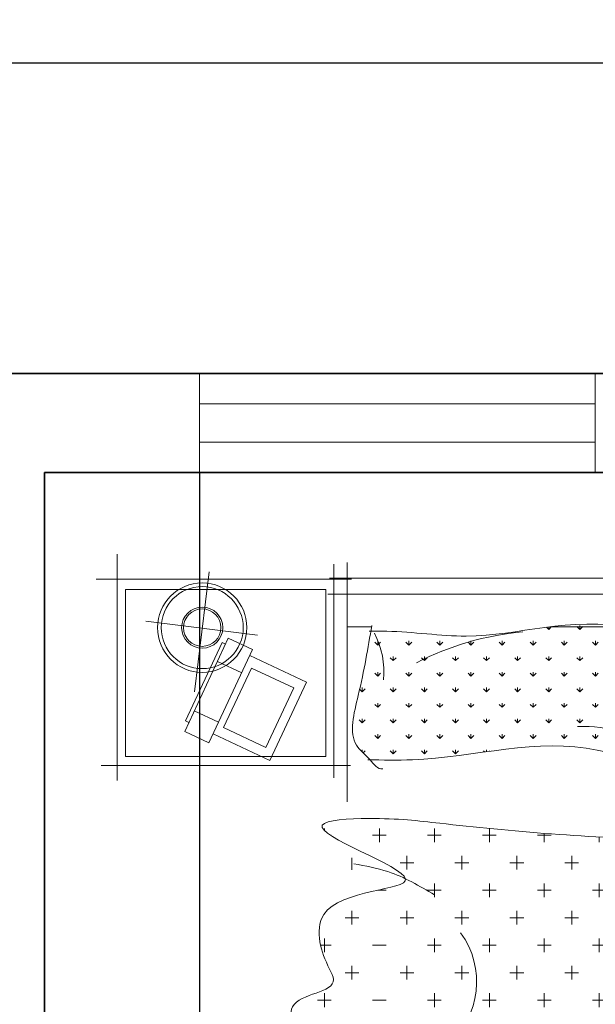
# Model space of a CAD drawing. Units: inches. Extents: x -26 to 575, y -18 to 513.
# Tile 13 of 28: x 136 to 189, y 418 to 508. Entities that reach past the tile are written whole.
import ezdxf

# ---------------------------------------------------------------- set-up
doc = ezdxf.new("R2010")
doc.units = ezdxf.units.IN
doc.header["$MEASUREMENT"] = 0
for name, color, linetype, lineweight in [('A-ANNO-DIMS', 2, 'Continuous', 18), ('A-GLAZ', 4, 'Continuous', 18), ('A-WALL', 7, 'Continuous', 35), ('Furniture', 8, 'Continuous', 15)]:
    doc.layers.add(name, color=color, linetype=linetype, lineweight=lineweight)
doc.styles.get("Standard").update_dxf_attribs({"font": 'arial.ttf', "height": 6})
doc.dimstyles.get("Standard").update_dxf_attribs({"dimtxt": 6, "dimasz": 0.18, "dimexe": 0.18, "dimexo": 0.0625, "dimgap": 0.09, "dimtad": 0, "dimtih": 1, "dimtoh": 1, "dimzin": 0, "dimdsep": 46, "dimlunit": 3, "dimtxsty": 'Standard', "dimcen": 0.09, "dimadec": 0, "dimazin": 0, "dimtfac": 1, "dimtofl": 0, "dimtmove": 0, "dimatfit": 3, "dimfxl": 1, "dimtolj": 1, "dimtzin": 0, "dimarcsym": 0})

# ---------------------------------------------------------------- blocks, each defined once
blk = doc.blocks.new('*D1')
at = {"layer": 'A-ANNO-DIMS', "color": 0, "lineweight": -2, "transparency": 16777216}
for p, q in [((18.177, 475.57), (18.177, 503.937)), ((18.357, 503.757), (264.875, 503.757)), ((521.997, 503.757), (275.479, 503.757)), ((522.177, 475.57), (522.177, 503.937))]:
    blk.add_line(p, q, dxfattribs=at)
at = {"layer": 'A-ANNO-DIMS', "color": 0, "transparency": 16777216}
for points in [[(18.357, 503.787), (18.357, 503.727), (18.177, 503.757)], [(521.997, 503.787), (521.997, 503.727), (522.177, 503.757)]]:
    blk.add_solid(points, dxfattribs=at)
at = {"layer": 'Defpoints', "color": 0, "transparency": 16777216}
for p in [(522.177, 503.757), (18.177, 475.508), (522.177, 475.508)]:
    blk.add_point(p, dxfattribs=at)
at = {"layer": 'A-ANNO-DIMS', "color": 0, "transparency": 16777216, "insert": (270.177, 503.757), "char_height": 6, "attachment_point": 5}
blk.add_mtext("\\A1;42'", dxfattribs=at)
blk = doc.blocks.new('BED-DOUBLE-WITH-NIGHTSTANDS')
for p, q in [((1.925, 83.361), (1.925, 62.761)), ((82.669, 83.361), (82.669, 62.761)), ((21.61, 63.031), (21.61, 82.461)), ((22.828, 60.828), (22.828, 82.615)), ((102.354, 63.031), (102.354, 82.461)), ((10.269, 81.761), (8.938, 70.826)), ((81.883, 82.344), (81.883, 56.232)), ((23.226, 81.078), (0, 81.078)), ((21.24, 81.17), (81.883, 81.17)), ((103.97, 81.078), (80.744, 81.078)), ((20.889, 80.153), (2.667, 80.153)), ((2.667, 80.153), (2.667, 64.968)), ((20.889, 64.968), (20.889, 80.153)), ((82.669, 79.717), (21.062, 79.717)), ((101.633, 80.153), (83.411, 80.153)), ((83.411, 80.153), (83.411, 64.968)), ((101.633, 64.968), (101.633, 80.153)), ((92.567, 79.403), (92.567, 67.508)), ((14.667, 76.005), (4.51, 77.257)), ((25.057, 76.764), (22.828, 76.764)), ((41.168, 76.507), (40.96, 76.715)), ((41.168, 76.507), (41.434, 76.772)), ((41.169, 76.507), (41.169, 76.741)), ((56.226, 76.764), (41.357, 76.764)), ((43.997, 76.507), (43.732, 76.772)), ((43.997, 76.507), (43.997, 76.882)), ((43.997, 76.507), (44.262, 76.772)), ((46.825, 76.507), (46.56, 76.772)), ((46.825, 76.507), (47.09, 76.772)), ((46.826, 76.507), (46.826, 76.882)), ((57.003, 76.507), (56.737, 76.772)), ((57.003, 76.507), (57.003, 76.828)), ((57.003, 76.507), (57.268, 76.772)), ((81.883, 76.764), (59.394, 76.764)), ((59.831, 76.507), (59.594, 76.744)), ((59.831, 76.507), (59.831, 76.717)), ((59.831, 76.507), (60.018, 76.694)), ((8.056, 67.244), (12.026, 75.725)), ((11.458, 75.323), (8.122, 68.196)), ((11.769, 75.177), (11.458, 75.323)), ((12.026, 75.725), (14.235, 74.691)), ((25.612, 75.093), (25.347, 75.358)), ((25.612, 75.093), (25.612, 75.468)), ((25.612, 75.093), (25.877, 75.358)), ((28.44, 75.093), (28.175, 75.358)), ((28.44, 75.093), (28.706, 75.358)), ((28.441, 75.093), (28.441, 75.468)), ((31.269, 75.093), (31.004, 75.358)), ((31.269, 75.093), (31.269, 75.468)), ((31.269, 75.093), (31.534, 75.358)), ((34.097, 75.093), (33.832, 75.358)), ((34.097, 75.093), (34.362, 75.358)), ((34.098, 75.093), (34.098, 75.468)), ((36.926, 75.093), (36.661, 75.358)), ((36.926, 75.093), (36.926, 75.468)), ((36.926, 75.093), (37.191, 75.358)), ((39.754, 75.093), (39.489, 75.358)), ((39.754, 75.093), (40.019, 75.358)), ((39.755, 75.093), (39.755, 75.468)), ((42.583, 75.093), (42.317, 75.358)), ((42.583, 75.093), (42.583, 75.468)), ((42.583, 75.093), (42.848, 75.358)), ((45.411, 75.093), (45.146, 75.358)), ((45.411, 75.093), (45.411, 75.468)), ((45.411, 75.093), (45.676, 75.358)), ((48.239, 75.093), (47.974, 75.358)), ((48.239, 75.093), (48.505, 75.358)), ((48.24, 75.093), (48.24, 75.468)), ((51.068, 75.093), (50.803, 75.358)), ((53.004, 75.337), (53.025, 75.358)), ((55.588, 75.093), (55.323, 75.358)), ((55.588, 75.093), (55.854, 75.358)), ((55.589, 75.093), (55.589, 75.468)), ((58.417, 75.093), (58.152, 75.358)), ((58.417, 75.093), (58.417, 75.468)), ((58.417, 75.093), (58.682, 75.358)), ((61.245, 75.093), (60.98, 75.358)), ((61.245, 75.093), (61.51, 75.358)), ((61.246, 75.093), (61.246, 75.468)), ((64.074, 75.093), (63.809, 75.358)), ((64.074, 75.093), (64.074, 75.468)), ((64.074, 75.093), (64.339, 75.358)), ((66.902, 75.093), (66.637, 75.358)), ((66.902, 75.093), (67.167, 75.358)), ((66.903, 75.093), (66.903, 75.468)), ((69.731, 75.093), (69.465, 75.358)), ((69.731, 75.093), (69.731, 75.468)), ((69.731, 75.093), (69.996, 75.358)), ((72.559, 75.093), (72.294, 75.358)), ((72.559, 75.093), (72.559, 75.468)), ((72.559, 75.093), (72.824, 75.358)), ((75.387, 75.093), (75.122, 75.358)), ((75.387, 75.093), (75.653, 75.358)), ((75.388, 75.093), (75.388, 75.468)), ((78.216, 75.093), (77.951, 75.358)), ((78.216, 75.093), (78.216, 75.468)), ((78.216, 75.093), (78.481, 75.358)), ((14.235, 74.691), (10.265, 66.21)), ((51.068, 75.093), (51.068, 75.099)), ((51.068, 75.093), (51.07, 75.095)), ((13.242, 72.571), (11.033, 73.605)), ((19.14, 71.727), (13.978, 74.143)), ((27.026, 73.679), (26.761, 73.944)), ((27.026, 73.679), (27.291, 73.944)), ((27.027, 73.678), (27.027, 74.053)), ((29.855, 73.679), (29.589, 73.944)), ((29.855, 73.678), (29.855, 74.053)), ((29.855, 73.679), (30.12, 73.944)), ((32.683, 73.679), (32.418, 73.944)), ((32.683, 73.678), (32.683, 74.053)), ((32.683, 73.679), (32.948, 73.944)), ((35.512, 73.679), (35.246, 73.944)), ((35.512, 73.678), (35.512, 74.053)), ((35.512, 73.679), (35.777, 73.944)), ((38.34, 73.679), (38.075, 73.944)), ((38.34, 73.678), (38.34, 74.053)), ((38.34, 73.679), (38.605, 73.944)), ((41.168, 73.679), (40.903, 73.944)), ((41.168, 73.679), (41.434, 73.944)), ((41.169, 73.678), (41.169, 74.053)), ((43.997, 73.679), (43.732, 73.944)), ((43.997, 73.678), (43.997, 74.053)), ((43.997, 73.679), (44.262, 73.944)), ((46.825, 73.679), (46.56, 73.944)), ((46.825, 73.679), (47.09, 73.944)), ((46.826, 73.678), (46.826, 74.053)), ((49.654, 73.679), (49.388, 73.944)), ((49.654, 73.678), (49.654, 74.053)), ((49.654, 73.679), (49.919, 73.944)), ((54.174, 73.679), (53.909, 73.944)), ((54.174, 73.679), (54.439, 73.944)), ((54.175, 73.678), (54.175, 74.053)), ((57.003, 73.679), (56.737, 73.944)), ((57.003, 73.678), (57.003, 74.053)), ((57.003, 73.679), (57.268, 73.944)), ((59.831, 73.679), (59.566, 73.944)), ((59.831, 73.678), (59.831, 74.053)), ((59.831, 73.679), (60.096, 73.944)), ((62.66, 73.679), (62.394, 73.944)), ((62.66, 73.678), (62.66, 74.053)), ((62.66, 73.679), (62.925, 73.944)), ((65.488, 73.679), (65.223, 73.944)), ((65.488, 73.678), (65.488, 74.053)), ((65.488, 73.679), (65.753, 73.944)), ((68.316, 73.679), (68.051, 73.944)), ((68.316, 73.679), (68.582, 73.944)), ((68.317, 73.678), (68.317, 74.053)), ((71.145, 73.679), (70.88, 73.944)), ((71.145, 73.678), (71.145, 74.053)), ((71.145, 73.679), (71.41, 73.944)), ((73.973, 73.679), (73.708, 73.944)), ((73.973, 73.679), (74.238, 73.944)), ((73.974, 73.678), (73.974, 74.053)), ((76.802, 73.679), (76.536, 73.944)), ((76.802, 73.678), (76.802, 74.053)), ((76.802, 73.679), (77.067, 73.944)), ((79.63, 73.679), (79.365, 73.944)), ((79.63, 73.678), (79.63, 74.053)), ((79.63, 73.679), (79.895, 73.944)), ((14.129, 73), (11.598, 67.591)), ((17.984, 71.195), (14.129, 73)), ((25.612, 72.264), (25.612, 72.639)), ((28.441, 72.264), (28.441, 72.639)), ((31.269, 72.264), (31.269, 72.639)), ((34.098, 72.264), (34.098, 72.639)), ((36.926, 72.264), (36.926, 72.639)), ((39.755, 72.264), (39.755, 72.639)), ((42.583, 72.264), (42.583, 72.639)), ((45.411, 72.264), (45.411, 72.639)), ((48.24, 72.264), (48.24, 72.639)), ((55.589, 72.264), (55.589, 72.639)), ((58.417, 72.264), (58.417, 72.639)), ((61.246, 72.264), (61.246, 72.639)), ((64.074, 72.264), (64.074, 72.639)), ((66.903, 72.264), (66.903, 72.639)), ((69.731, 72.264), (69.731, 72.639)), ((72.559, 72.264), (72.559, 72.639)), ((75.388, 72.264), (75.388, 72.639)), ((78.216, 72.264), (78.216, 72.639)), ((98.466, 73.144), (86.668, 73.144)), ((15.804, 64.601), (19.14, 71.727)), ((25.612, 72.265), (25.347, 72.53)), ((25.612, 72.265), (25.877, 72.53)), ((28.44, 72.265), (28.175, 72.53)), ((28.44, 72.265), (28.706, 72.53)), ((31.269, 72.265), (31.004, 72.53)), ((31.269, 72.265), (31.534, 72.53)), ((34.097, 72.265), (33.832, 72.53)), ((34.097, 72.265), (34.362, 72.53)), ((36.926, 72.265), (36.661, 72.53)), ((36.926, 72.265), (37.191, 72.53)), ((39.754, 72.265), (39.489, 72.53)), ((39.754, 72.265), (40.019, 72.53)), ((42.583, 72.265), (42.317, 72.53)), ((42.583, 72.265), (42.848, 72.53)), ((45.411, 72.265), (45.146, 72.53)), ((45.411, 72.265), (45.676, 72.53)), ((48.239, 72.265), (47.974, 72.53)), ((48.239, 72.265), (48.505, 72.53)), ((55.588, 72.265), (55.323, 72.53)), ((55.588, 72.265), (55.854, 72.53)), ((58.417, 72.265), (58.152, 72.53)), ((58.417, 72.265), (58.682, 72.53)), ((61.245, 72.265), (60.98, 72.53)), ((61.245, 72.265), (61.51, 72.53)), ((64.074, 72.265), (63.809, 72.53)), ((64.074, 72.265), (64.339, 72.53)), ((66.902, 72.265), (66.637, 72.53)), ((66.902, 72.265), (67.167, 72.53)), ((69.731, 72.265), (69.465, 72.53)), ((69.731, 72.265), (69.996, 72.53)), ((72.559, 72.265), (72.294, 72.53)), ((72.559, 72.265), (72.824, 72.53)), ((75.387, 72.265), (75.122, 72.53)), ((75.387, 72.265), (75.653, 72.53)), ((78.216, 72.265), (77.951, 72.53)), ((78.216, 72.265), (78.481, 72.53)), ((15.452, 65.787), (17.984, 71.195)), ((24.198, 70.85), (23.972, 71.076)), ((24.198, 70.85), (24.198, 71.225)), ((24.198, 70.85), (24.463, 71.116)), ((27.026, 70.85), (26.761, 71.116)), ((27.026, 70.85), (27.291, 71.116)), ((27.027, 70.85), (27.027, 71.225)), ((29.855, 70.85), (29.589, 71.116)), ((29.855, 70.85), (29.855, 71.225)), ((29.855, 70.85), (30.12, 71.116)), ((32.683, 70.85), (32.418, 71.116)), ((32.683, 70.85), (32.683, 71.225)), ((32.683, 70.85), (32.948, 71.116)), ((35.512, 70.85), (35.246, 71.116)), ((35.512, 70.85), (35.512, 71.225)), ((35.512, 70.85), (35.777, 71.116)), ((38.34, 70.85), (38.075, 71.116)), ((38.34, 70.85), (38.34, 71.225)), ((38.34, 70.85), (38.605, 71.116)), ((41.168, 70.85), (40.903, 71.116)), ((41.168, 70.85), (41.434, 71.116)), ((41.169, 70.85), (41.169, 71.225)), ((43.997, 70.85), (43.732, 71.116)), ((43.997, 70.85), (43.997, 71.225)), ((43.997, 70.85), (44.262, 71.116)), ((46.825, 70.85), (46.56, 71.116)), ((46.825, 70.85), (47.09, 71.116)), ((46.826, 70.85), (46.826, 71.225)), ((49.654, 70.85), (49.388, 71.116)), ((49.654, 70.85), (49.654, 71.225)), ((49.654, 70.85), (49.919, 71.116)), ((54.174, 70.85), (53.909, 71.116)), ((54.174, 70.85), (54.439, 71.116)), ((54.175, 70.85), (54.175, 71.225)), ((57.003, 70.85), (56.737, 71.116)), ((57.003, 70.85), (57.003, 71.225)), ((57.003, 70.85), (57.268, 71.116)), ((59.831, 70.85), (59.566, 71.116)), ((59.831, 70.85), (59.831, 71.225)), ((59.831, 70.85), (60.096, 71.116)), ((62.66, 70.85), (62.394, 71.116)), ((62.66, 70.85), (62.66, 71.225)), ((62.66, 70.85), (62.925, 71.116)), ((65.488, 70.85), (65.223, 71.116)), ((65.488, 70.85), (65.488, 71.225)), ((65.488, 70.85), (65.753, 71.116)), ((68.316, 70.85), (68.051, 71.116)), ((68.316, 70.85), (68.582, 71.116)), ((68.317, 70.85), (68.317, 71.225)), ((71.145, 70.85), (70.88, 71.116)), ((71.145, 70.85), (71.145, 71.225)), ((71.145, 70.85), (71.41, 71.116)), ((73.973, 70.85), (73.708, 71.116)), ((73.973, 70.85), (74.238, 71.116)), ((73.974, 70.85), (73.974, 71.225)), ((76.802, 70.85), (76.536, 71.116)), ((76.802, 70.85), (76.802, 71.225)), ((76.802, 70.85), (77.067, 71.116)), ((79.63, 70.85), (79.365, 71.116)), ((79.63, 70.85), (79.63, 71.225)), ((79.63, 70.85), (79.895, 71.116)), ((11.136, 68.071), (8.927, 69.105)), ((25.612, 69.436), (25.347, 69.701)), ((25.612, 69.436), (25.612, 69.811)), ((25.612, 69.436), (25.877, 69.701)), ((28.44, 69.436), (28.175, 69.701)), ((28.44, 69.436), (28.706, 69.701)), ((28.441, 69.436), (28.441, 69.811)), ((31.269, 69.436), (31.004, 69.701)), ((31.269, 69.436), (31.269, 69.811)), ((31.269, 69.436), (31.534, 69.701)), ((34.097, 69.436), (33.832, 69.701)), ((34.097, 69.436), (34.362, 69.701)), ((34.098, 69.436), (34.098, 69.811)), ((36.926, 69.436), (36.661, 69.701)), ((36.926, 69.436), (36.926, 69.811)), ((36.926, 69.436), (37.191, 69.701)), ((39.754, 69.436), (39.489, 69.701)), ((39.754, 69.436), (40.019, 69.701)), ((39.755, 69.436), (39.755, 69.811)), ((42.583, 69.436), (42.317, 69.701)), ((42.583, 69.436), (42.583, 69.811)), ((42.583, 69.436), (42.848, 69.701)), ((45.411, 69.436), (45.146, 69.701)), ((45.411, 69.436), (45.411, 69.811)), ((45.411, 69.436), (45.676, 69.701)), ((48.239, 69.436), (47.974, 69.701)), ((48.239, 69.436), (48.505, 69.701)), ((48.24, 69.436), (48.24, 69.811)), ((51.052, 69.452), (50.803, 69.701)), ((53.007, 69.683), (53.025, 69.701)), ((55.588, 69.436), (55.323, 69.701)), ((55.588, 69.436), (55.854, 69.701)), ((55.589, 69.436), (55.589, 69.811)), ((58.417, 69.436), (58.152, 69.701)), ((58.417, 69.436), (58.417, 69.811)), ((58.417, 69.436), (58.682, 69.701)), ((61.245, 69.436), (60.98, 69.701)), ((61.245, 69.436), (61.51, 69.701)), ((61.246, 69.436), (61.246, 69.811)), ((64.074, 69.436), (63.809, 69.701)), ((64.074, 69.436), (64.074, 69.811)), ((64.074, 69.436), (64.339, 69.701)), ((66.902, 69.436), (66.637, 69.701)), ((66.902, 69.436), (67.167, 69.701)), ((66.903, 69.436), (66.903, 69.811)), ((69.731, 69.436), (69.465, 69.701)), ((69.731, 69.436), (69.731, 69.811)), ((69.731, 69.436), (69.996, 69.701)), ((72.559, 69.436), (72.294, 69.701)), ((72.559, 69.436), (72.559, 69.811)), ((72.559, 69.436), (72.824, 69.701)), ((75.387, 69.436), (75.122, 69.701)), ((75.387, 69.436), (75.653, 69.701)), ((75.388, 69.436), (75.388, 69.811)), ((78.216, 69.436), (77.951, 69.701)), ((78.216, 69.436), (78.216, 69.811)), ((78.216, 69.436), (78.481, 69.701)), ((8.122, 68.196), (8.434, 68.05)), ((24.198, 68.022), (23.933, 68.287)), ((24.198, 68.022), (24.198, 68.397)), ((24.198, 68.022), (24.463, 68.287)), ((27.026, 68.022), (26.761, 68.287)), ((27.026, 68.022), (27.291, 68.287)), ((27.027, 68.022), (27.027, 68.397)), ((29.855, 68.022), (29.589, 68.287)), ((29.855, 68.022), (29.855, 68.397)), ((29.855, 68.022), (30.12, 68.287)), ((32.683, 68.022), (32.418, 68.287)), ((32.683, 68.022), (32.683, 68.397)), ((32.683, 68.022), (32.948, 68.287)), ((35.512, 68.022), (35.246, 68.287)), ((35.512, 68.022), (35.512, 68.397)), ((35.512, 68.022), (35.777, 68.287)), ((38.34, 68.022), (38.075, 68.287)), ((38.34, 68.022), (38.34, 68.397)), ((38.34, 68.022), (38.605, 68.287)), ((41.168, 68.022), (40.903, 68.287)), ((41.168, 68.022), (41.434, 68.287)), ((41.169, 68.022), (41.169, 68.397)), ((43.997, 68.022), (43.732, 68.287)), ((43.997, 68.022), (43.997, 68.397)), ((43.997, 68.022), (44.262, 68.287)), ((46.825, 68.022), (46.56, 68.287)), ((46.825, 68.022), (47.09, 68.287)), ((46.826, 68.022), (46.826, 68.397)), ((49.654, 68.022), (49.388, 68.287)), ((49.654, 68.022), (49.654, 68.397)), ((49.654, 68.022), (49.919, 68.287)), ((54.174, 68.022), (53.909, 68.287)), ((54.174, 68.022), (54.439, 68.287)), ((54.175, 68.022), (54.175, 68.397)), ((57.003, 68.022), (56.737, 68.287)), ((57.003, 68.022), (57.003, 68.397)), ((57.003, 68.022), (57.268, 68.287)), ((59.831, 68.022), (59.566, 68.287)), ((59.831, 68.022), (59.831, 68.397)), ((59.831, 68.022), (60.096, 68.287)), ((62.66, 68.022), (62.394, 68.287)), ((62.66, 68.022), (62.66, 68.397)), ((62.66, 68.022), (62.925, 68.287)), ((65.488, 68.022), (65.223, 68.287)), ((65.488, 68.022), (65.488, 68.397)), ((65.488, 68.022), (65.753, 68.287)), ((68.316, 68.022), (68.051, 68.287)), ((68.316, 68.022), (68.582, 68.287)), ((68.317, 68.022), (68.317, 68.397)), ((71.145, 68.022), (70.88, 68.287)), ((71.145, 68.022), (71.145, 68.397)), ((71.145, 68.022), (71.41, 68.287)), ((73.973, 68.022), (73.708, 68.287)), ((73.973, 68.022), (74.238, 68.287)), ((73.974, 68.022), (73.974, 68.397)), ((76.802, 68.022), (76.536, 68.287)), ((76.802, 68.022), (76.802, 68.397)), ((76.802, 68.022), (77.067, 68.287)), ((79.63, 68.022), (79.365, 68.287)), ((79.63, 68.022), (79.63, 68.397)), ((79.63, 68.022), (79.895, 68.287)), ((10.265, 66.21), (8.056, 67.244)), ((11.598, 67.591), (15.452, 65.787)), ((10.642, 67.017), (15.804, 64.601)), ((25.612, 66.608), (25.347, 66.873)), ((25.612, 66.607), (25.612, 66.982)), ((25.612, 66.608), (25.877, 66.873)), ((28.44, 66.608), (28.175, 66.873)), ((28.44, 66.608), (28.706, 66.873)), ((28.441, 66.607), (28.441, 66.982)), ((31.269, 66.608), (31.004, 66.873)), ((31.269, 66.607), (31.269, 66.982)), ((31.269, 66.608), (31.534, 66.873)), ((34.097, 66.608), (33.832, 66.873)), ((34.097, 66.608), (34.362, 66.873)), ((34.098, 66.607), (34.098, 66.982)), ((36.926, 66.608), (36.661, 66.873)), ((36.926, 66.607), (36.926, 66.982)), ((36.926, 66.608), (37.191, 66.873)), ((39.754, 66.608), (39.489, 66.873)), ((39.754, 66.608), (40.019, 66.873)), ((39.755, 66.607), (39.755, 66.982)), ((42.583, 66.608), (42.317, 66.873)), ((42.583, 66.607), (42.583, 66.982)), ((42.583, 66.608), (42.848, 66.873)), ((45.411, 66.608), (45.146, 66.873)), ((45.411, 66.607), (45.411, 66.982)), ((45.411, 66.608), (45.676, 66.873)), ((48.239, 66.608), (47.974, 66.873)), ((48.239, 66.608), (48.505, 66.873)), ((48.24, 66.607), (48.24, 66.982)), ((51.068, 66.608), (50.803, 66.873)), ((51.068, 66.607), (51.068, 66.982)), ((51.068, 66.608), (51.333, 66.873)), ((52.76, 66.608), (52.495, 66.873)), ((52.76, 66.607), (52.76, 66.982)), ((52.76, 66.608), (53.025, 66.873)), ((55.588, 66.608), (55.323, 66.873)), ((55.588, 66.608), (55.854, 66.873)), ((55.589, 66.607), (55.589, 66.982)), ((58.417, 66.608), (58.152, 66.873)), ((58.417, 66.607), (58.417, 66.982)), ((58.417, 66.608), (58.682, 66.873)), ((61.245, 66.608), (60.98, 66.873)), ((61.245, 66.608), (61.51, 66.873)), ((61.246, 66.607), (61.246, 66.982)), ((64.074, 66.608), (63.809, 66.873)), ((64.074, 66.607), (64.074, 66.982)), ((64.074, 66.608), (64.339, 66.873)), ((66.902, 66.608), (66.637, 66.873)), ((66.902, 66.608), (67.167, 66.873)), ((66.903, 66.607), (66.903, 66.982)), ((69.731, 66.608), (69.465, 66.873)), ((69.731, 66.607), (69.731, 66.982)), ((69.731, 66.608), (69.996, 66.873)), ((72.559, 66.608), (72.294, 66.873)), ((72.559, 66.607), (72.559, 66.982)), ((72.559, 66.608), (72.824, 66.873)), ((75.387, 66.608), (75.122, 66.873)), ((75.387, 66.608), (75.653, 66.873)), ((75.388, 66.607), (75.388, 66.982)), ((78.216, 66.608), (77.951, 66.873)), ((78.216, 66.607), (78.216, 66.982)), ((78.216, 66.608), (78.481, 66.873)), ((81.044, 66.608), (80.779, 66.873)), ((81.044, 66.608), (81.253, 66.817)), ((81.045, 66.607), (81.045, 66.982)), ((24.198, 65.385), (24.198, 65.568)), ((24.295, 65.291), (24.463, 65.459)), ((27.026, 65.194), (26.761, 65.459)), ((27.026, 65.194), (27.291, 65.459)), ((27.027, 65.193), (27.027, 65.568)), ((29.855, 65.194), (29.589, 65.459)), ((29.855, 65.193), (29.855, 65.568)), ((29.855, 65.194), (30.12, 65.459)), ((32.683, 65.194), (32.418, 65.459)), ((32.683, 65.193), (32.683, 65.568)), ((32.683, 65.194), (32.948, 65.459)), ((35.335, 65.37), (35.246, 65.459)), ((35.512, 65.394), (35.512, 65.568)), ((35.743, 65.425), (35.777, 65.459)), ((46.774, 65.245), (46.56, 65.459)), ((46.826, 65.232), (46.826, 65.568)), ((46.856, 65.224), (47.09, 65.459)), ((49.654, 65.194), (49.388, 65.459)), ((49.654, 65.193), (49.654, 65.568)), ((49.654, 65.194), (49.919, 65.459)), ((54.174, 65.194), (53.909, 65.459)), ((54.174, 65.194), (54.439, 65.459)), ((54.175, 65.193), (54.175, 65.568)), ((57.003, 65.194), (56.737, 65.459)), ((57.003, 65.193), (57.003, 65.568)), ((57.003, 65.194), (57.268, 65.459)), ((59.831, 65.194), (59.566, 65.459)), ((59.831, 65.193), (59.831, 65.568)), ((59.831, 65.194), (60.096, 65.459)), ((62.66, 65.525), (62.66, 65.568)), ((65.488, 65.481), (65.488, 65.568)), ((65.74, 65.446), (65.753, 65.459)), ((68.316, 65.194), (68.051, 65.459)), ((68.316, 65.194), (68.582, 65.459)), ((68.317, 65.193), (68.317, 65.568)), ((71.145, 65.194), (70.88, 65.459)), ((71.145, 65.193), (71.145, 65.568)), ((71.145, 65.194), (71.41, 65.459)), ((73.973, 65.194), (73.708, 65.459)), ((73.973, 65.194), (74.238, 65.459)), ((73.974, 65.193), (73.974, 65.568)), ((76.802, 65.194), (76.536, 65.459)), ((76.802, 65.193), (76.802, 65.568)), ((76.802, 65.194), (77.067, 65.459)), ((79.63, 65.194), (79.365, 65.459)), ((79.63, 65.193), (79.63, 65.568)), ((79.63, 65.194), (79.895, 65.459)), ((82.154, 61.735), (82.154, 65.422)), ((2.667, 64.968), (20.889, 64.968)), ((83.411, 64.968), (101.633, 64.968)), ((0.451, 64.149), (23.136, 64.149)), ((55.589, 64.121), (55.589, 64.154)), ((81.194, 64.149), (103.88, 64.149)), ((78.267, 59.667), (78.267, 60.149)), ((20.767, 58.212), (20.767, 58.417)), ((25.767, 57.167), (25.767, 58.417)), ((30.767, 57.167), (30.767, 58.417)), ((35.767, 57.167), (35.767, 58.407)), ((70.767, 57.167), (70.767, 58.417)), ((75.767, 57.167), (75.767, 58.417)), ((80.767, 57.167), (80.767, 58.417)), ((21.392, 57.792), (21.312, 57.792)), ((26.392, 57.792), (25.142, 57.792)), ((31.392, 57.792), (30.142, 57.792)), ((36.392, 57.792), (35.142, 57.792)), ((41.392, 57.792), (40.142, 57.792)), ((40.767, 57.167), (40.767, 57.965)), ((45.767, 57.167), (45.767, 57.639)), ((50.767, 57.167), (50.767, 57.462)), ((55.767, 57.167), (55.767, 57.483)), ((60.767, 57.167), (60.767, 57.735)), ((66.392, 57.792), (65.142, 57.792)), ((65.767, 57.167), (65.767, 58.213)), ((71.392, 57.792), (70.142, 57.792)), ((76.392, 57.792), (75.142, 57.792)), ((81.392, 57.792), (80.142, 57.792)), ((23.273, 54.636), (23.273, 55.755)), ((28.267, 54.667), (28.267, 55.917)), ((33.267, 54.667), (33.267, 55.917)), ((38.267, 54.667), (38.267, 55.917)), ((43.267, 54.667), (43.267, 55.917)), ((48.267, 54.667), (48.267, 55.917)), ((53.267, 54.667), (53.267, 55.917)), ((58.267, 54.667), (58.267, 55.917)), ((63.267, 54.667), (63.267, 55.917)), ((68.267, 54.667), (68.267, 55.917)), ((73.267, 54.667), (73.267, 55.917)), ((78.267, 54.667), (78.267, 55.917)), ((83.267, 54.667), (83.267, 55.917)), ((28.892, 55.292), (27.642, 55.292)), ((33.892, 55.292), (32.642, 55.292)), ((38.892, 55.292), (37.642, 55.292)), ((43.892, 55.292), (42.642, 55.292)), ((48.892, 55.292), (47.642, 55.292)), ((53.892, 55.292), (52.642, 55.292)), ((58.892, 55.292), (57.642, 55.292)), ((63.892, 55.292), (62.642, 55.292)), ((68.892, 55.292), (67.642, 55.292)), ((73.892, 55.292), (72.642, 55.292)), ((78.892, 55.292), (77.642, 55.292)), ((83.892, 55.292), (82.642, 55.292)), ((30.767, 52.167), (30.767, 53.417)), ((35.767, 52.167), (35.767, 53.417)), ((40.767, 52.167), (40.767, 53.417)), ((45.767, 52.167), (45.767, 53.417)), ((50.767, 52.167), (50.767, 53.417)), ((55.767, 52.167), (55.767, 53.417)), ((60.767, 52.167), (60.767, 53.417)), ((65.767, 52.167), (65.767, 53.417)), ((70.767, 52.167), (70.767, 53.417)), ((75.767, 52.167), (75.767, 53.417)), ((80.767, 52.167), (80.767, 53.417)), ((26.392, 52.792), (25.619, 52.792)), ((31.392, 52.792), (30.142, 52.792)), ((36.392, 52.792), (35.142, 52.792)), ((41.392, 52.792), (40.142, 52.792)), ((46.392, 52.792), (45.142, 52.792)), ((51.392, 52.792), (50.142, 52.792)), ((56.392, 52.792), (55.142, 52.792)), ((61.392, 52.792), (60.142, 52.792)), ((66.392, 52.792), (65.142, 52.792)), ((71.392, 52.792), (70.142, 52.792)), ((76.392, 52.792), (75.142, 52.792)), ((81.392, 52.792), (80.142, 52.792)), ((23.892, 50.292), (22.642, 50.292)), ((23.267, 49.667), (23.267, 50.917)), ((28.892, 50.292), (27.642, 50.292)), ((28.267, 49.667), (28.267, 50.917)), ((33.892, 50.292), (32.642, 50.292)), ((33.267, 49.667), (33.267, 50.917)), ((38.892, 50.292), (37.642, 50.292)), ((38.267, 49.667), (38.267, 50.917)), ((43.892, 50.292), (42.642, 50.292)), ((43.267, 49.667), (43.267, 50.917)), ((48.892, 50.292), (47.642, 50.292)), ((48.267, 49.667), (48.267, 50.917)), ((53.892, 50.292), (52.642, 50.292)), ((53.267, 49.667), (53.267, 50.917)), ((58.892, 50.292), (57.642, 50.292)), ((58.267, 49.667), (58.267, 50.917)), ((63.892, 50.292), (62.642, 50.292)), ((63.267, 49.667), (63.267, 50.917)), ((68.892, 50.292), (67.642, 50.292)), ((68.267, 49.667), (68.267, 50.917)), ((73.892, 50.292), (72.642, 50.292)), ((73.267, 49.667), (73.267, 50.917)), ((78.892, 50.292), (77.642, 50.292)), ((78.267, 49.667), (78.267, 50.917)), ((83.892, 50.292), (82.642, 50.292)), ((83.267, 49.667), (83.267, 50.917)), ((20.767, 47.167), (20.767, 48.417)), ((30.767, 47.167), (30.767, 48.417)), ((35.767, 47.167), (35.767, 48.417)), ((40.767, 47.167), (40.767, 48.417)), ((45.767, 47.167), (45.767, 48.417)), ((50.767, 47.167), (50.767, 48.417)), ((55.767, 47.167), (55.767, 48.417)), ((65.767, 47.167), (65.767, 48.417)), ((70.767, 47.167), (70.767, 48.417)), ((75.767, 47.167), (75.767, 48.417)), ((80.767, 47.167), (80.767, 48.417)), ((21.392, 47.792), (20.412, 47.792)), ((26.392, 47.792), (25.142, 47.792)), ((31.392, 47.792), (30.142, 47.792)), ((36.392, 47.792), (35.142, 47.792)), ((41.392, 47.792), (40.142, 47.792)), ((46.392, 47.792), (45.142, 47.792)), ((51.392, 47.792), (50.142, 47.792)), ((56.392, 47.792), (55.142, 47.792)), ((66.392, 47.792), (65.142, 47.792)), ((71.392, 47.792), (70.142, 47.792)), ((76.392, 47.792), (75.142, 47.792)), ((81.392, 47.792), (80.142, 47.792)), ((23.267, 44.667), (23.267, 45.917)), ((28.267, 44.667), (28.267, 45.917)), ((33.267, 44.667), (33.267, 45.917)), ((38.267, 44.667), (38.267, 45.917)), ((43.267, 44.667), (43.267, 45.917)), ((48.267, 44.667), (48.267, 45.917)), ((53.267, 44.667), (53.267, 45.917)), ((63.267, 44.667), (63.267, 45.917)), ((68.267, 44.667), (68.267, 45.917)), ((73.267, 44.667), (73.267, 45.917)), ((78.267, 44.667), (78.267, 45.917)), ((83.267, 44.667), (83.267, 45.917)), ((23.892, 45.292), (22.642, 45.292)), ((28.892, 45.292), (27.642, 45.292)), ((33.892, 45.292), (32.642, 45.292)), ((38.892, 45.292), (37.642, 45.292)), ((43.892, 45.292), (42.642, 45.292)), ((48.892, 45.292), (47.642, 45.292)), ((53.892, 45.292), (52.642, 45.292)), ((58.892, 45.292), (57.642, 45.292)), ((63.892, 45.292), (62.642, 45.292)), ((68.892, 45.292), (67.642, 45.292)), ((73.892, 45.292), (72.642, 45.292)), ((78.892, 45.292), (77.642, 45.292)), ((83.892, 45.292), (82.642, 45.292)), ((20.767, 42.167), (20.767, 43.417)), ((30.767, 42.167), (30.767, 43.417)), ((35.767, 42.167), (35.767, 43.417)), ((40.767, 42.167), (40.767, 43.417)), ((45.767, 42.167), (45.767, 43.417)), ((50.767, 42.167), (50.767, 43.417)), ((55.767, 42.167), (55.767, 43.417)), ((65.767, 42.167), (65.767, 43.417)), ((70.767, 42.167), (70.767, 43.417)), ((75.767, 42.167), (75.767, 43.417)), ((80.767, 42.167), (80.767, 43.417)), ((85.767, 42.167), (85.767, 43.417)), ((21.392, 42.792), (20.142, 42.792)), ((26.392, 42.792), (25.142, 42.792)), ((31.392, 42.792), (30.142, 42.792)), ((36.392, 42.792), (35.142, 42.792)), ((41.392, 42.792), (40.142, 42.792)), ((46.392, 42.792), (45.142, 42.792)), ((51.392, 42.792), (50.142, 42.792)), ((56.392, 42.792), (55.142, 42.792)), ((61.392, 42.792), (60.142, 42.792)), ((66.089, 42.792), (65.142, 42.792)), ((72.149, 42.386), (71.41, 42.386)), ((71.779, 42.017), (71.779, 42.495)), ((76.392, 42.792), (76.07, 42.792)), ((81.392, 42.792), (80.142, 42.792)), ((81.883, 42.36), (81.883, 0)), ((86.392, 42.792), (85.142, 42.792)), ((70.303, 40.541), (70.303, 41.279)), ((73.256, 40.541), (73.256, 41.279)), ((18.267, 39.667), (18.267, 40.917)), ((23.267, 39.991), (23.267, 40.917)), ((28.267, 39.667), (28.267, 40.917)), ((33.267, 39.667), (33.267, 40.917)), ((38.267, 39.667), (38.267, 40.917)), ((43.267, 39.667), (43.267, 40.917)), ((48.267, 39.667), (48.267, 40.917)), ((53.267, 39.667), (53.267, 40.917)), ((63.267, 39.667), (63.267, 40.917)), ((67.35, 40.541), (67.35, 40.835)), ((67.719, 40.91), (67.48, 40.91)), ((68.267, 39.667), (68.267, 40.917)), ((70.672, 40.91), (69.934, 40.91)), ((73.625, 40.91), (72.887, 40.91)), ((73.267, 39.667), (73.267, 40.917)), ((76.578, 40.91), (75.839, 40.91)), ((76.209, 40.541), (76.209, 41.133)), ((78.267, 39.667), (78.267, 40.917)), ((83.267, 39.667), (83.267, 40.917)), ((18.892, 40.292), (17.831, 40.292)), ((23.892, 40.292), (22.642, 40.292)), ((28.892, 40.292), (27.642, 40.292)), ((33.892, 40.292), (32.642, 40.292)), ((38.892, 40.292), (37.642, 40.292)), ((43.892, 40.292), (42.642, 40.292)), ((48.892, 40.292), (47.642, 40.292)), ((53.892, 40.292), (52.642, 40.292)), ((58.892, 40.292), (57.642, 40.292)), ((62.901, 40.292), (62.642, 40.292)), ((66.243, 39.433), (65.505, 39.433)), ((65.874, 39.064), (65.874, 39.802)), ((69.196, 39.433), (68.458, 39.433)), ((68.827, 39.064), (68.827, 39.802)), ((72.149, 39.433), (71.41, 39.433)), ((71.779, 39.064), (71.779, 39.802)), ((75.101, 39.433), (74.363, 39.433)), ((74.732, 39.064), (74.732, 39.802)), ((78.054, 39.433), (77.316, 39.433)), ((77.685, 39.064), (77.685, 39.802)), ((83.892, 40.292), (82.642, 40.292)), ((22.828, 3.418), (22.828, 38.865)), ((25.767, 37.167), (25.767, 38.417)), ((30.767, 37.167), (30.767, 38.417)), ((35.767, 37.167), (35.767, 38.417)), ((40.767, 37.167), (40.767, 38.417)), ((45.767, 37.167), (45.767, 38.417)), ((50.767, 37.167), (50.767, 38.417)), ((55.767, 37.167), (55.767, 38.417)), ((61.392, 37.792), (60.142, 37.792)), ((60.767, 37.167), (60.767, 38.417)), ((64.767, 37.957), (64.028, 37.957)), ((64.398, 37.588), (64.398, 38.326)), ((66.392, 37.792), (65.142, 37.792)), ((65.767, 37.167), (65.767, 38.417)), ((67.719, 37.957), (66.981, 37.957)), ((67.35, 37.588), (67.35, 38.326)), ((70.672, 37.957), (69.934, 37.957)), ((71.392, 37.792), (70.142, 37.792)), ((70.303, 37.588), (70.303, 38.326)), ((70.767, 37.167), (70.767, 38.417)), ((73.625, 37.957), (72.887, 37.957)), ((73.256, 37.588), (73.256, 38.326)), ((76.392, 37.792), (75.142, 37.792)), ((75.767, 37.167), (75.767, 38.417)), ((76.451, 37.957), (75.839, 37.957)), ((76.209, 37.798), (76.209, 38.326)), ((81.392, 37.792), (80.142, 37.792)), ((80.767, 37.167), (80.767, 38.417)), ((62.921, 36.111), (62.921, 36.85)), ((65.874, 36.111), (65.874, 36.85)), ((68.827, 36.111), (68.827, 36.85)), ((71.779, 36.111), (71.779, 36.85)), ((74.732, 36.661), (74.732, 36.85)), ((28.267, 34.667), (28.267, 35.917)), ((33.267, 34.667), (33.267, 35.917)), ((38.267, 34.667), (38.267, 35.917)), ((43.267, 34.667), (43.267, 35.917)), ((48.267, 34.667), (48.267, 35.917)), ((53.267, 34.667), (53.267, 35.917)), ((58.267, 34.667), (58.267, 35.917)), ((59.968, 36.111), (59.968, 36.158)), ((63.29, 36.481), (62.552, 36.481)), ((63.267, 34.667), (63.267, 35.917)), ((66.243, 36.481), (65.505, 36.481)), ((68.267, 34.667), (68.267, 35.917)), ((69.196, 36.481), (68.458, 36.481)), ((72.149, 36.481), (71.41, 36.481)), ((73.267, 34.667), (73.267, 35.917)), ((74.53, 36.481), (74.363, 36.481)), ((78.267, 34.667), (78.267, 35.917)), ((17.658, 35.292), (17.642, 35.292)), ((58.892, 35.292), (57.642, 35.292)), ((58.861, 35.004), (58.123, 35.004)), ((58.492, 34.635), (58.492, 35.373)), ((61.814, 35.004), (61.076, 35.004)), ((61.445, 34.635), (61.445, 35.373)), ((63.892, 35.292), (62.642, 35.292)), ((64.767, 35.004), (64.028, 35.004)), ((64.398, 34.635), (64.398, 35.373)), ((67.719, 35.004), (66.981, 35.004)), ((67.35, 34.635), (67.35, 35.373)), ((68.892, 35.292), (67.642, 35.292)), ((70.672, 35.004), (69.934, 35.004)), ((70.303, 34.635), (70.303, 35.373)), ((73.892, 35.292), (72.642, 35.292)), ((73.008, 35.004), (72.887, 35.004)), ((73.256, 35.252), (73.256, 35.373)), ((78.892, 35.292), (77.642, 35.292)), ((25.767, 32.167), (25.767, 33.417)), ((30.767, 32.167), (30.767, 33.417)), ((35.767, 32.167), (35.767, 33.417)), ((40.767, 32.167), (40.767, 33.417)), ((45.767, 32.167), (45.767, 33.417)), ((50.767, 32.167), (50.767, 33.417)), ((51.11, 33.245), (51.11, 33.484)), ((54.432, 33.528), (53.694, 33.528)), ((54.063, 33.159), (54.063, 33.897)), ((55.767, 32.167), (55.767, 33.417)), ((57.385, 33.528), (56.647, 33.528)), ((57.016, 33.159), (57.016, 33.897)), ((60.338, 33.528), (59.599, 33.528)), ((59.968, 33.159), (59.968, 33.897)), ((60.767, 32.167), (60.767, 33.417)), ((63.29, 33.528), (62.552, 33.528)), ((62.921, 33.159), (62.921, 33.897)), ((66.243, 33.528), (65.505, 33.528)), ((65.767, 32.167), (65.767, 33.417)), ((65.874, 33.159), (65.874, 33.897)), ((69.196, 33.528), (68.458, 33.528)), ((68.827, 33.159), (68.827, 33.897)), ((70.767, 32.167), (70.767, 33.417)), ((71.469, 33.528), (71.41, 33.528)), ((71.779, 33.808), (71.779, 33.897)), ((75.767, 32.167), (75.767, 33.417)), ((80.767, 32.167), (80.767, 33.417)), ((55.539, 32.371), (55.539, 32.421)), ((58.492, 31.744), (58.492, 32.421)), ((61.445, 31.682), (61.445, 32.421)), ((64.398, 31.682), (64.398, 32.421)), ((67.35, 31.682), (67.35, 32.421)), ((58.861, 32.051), (58.123, 32.051)), ((61.814, 32.051), (61.076, 32.051)), ((64.767, 32.051), (64.028, 32.051)), ((67.719, 32.051), (66.981, 32.051)), ((28.267, 29.667), (28.267, 30.917)), ((33.267, 29.667), (33.267, 30.917)), ((38.267, 29.667), (38.267, 30.917)), ((43.267, 29.667), (43.267, 30.917)), ((48.267, 29.667), (48.267, 30.917)), ((53.267, 29.667), (53.267, 30.917)), ((58.267, 29.667), (58.267, 30.917)), ((63.267, 29.667), (63.267, 30.917)), ((68.267, 29.667), (68.267, 30.917)), ((73.267, 29.667), (73.267, 30.917)), ((78.267, 29.667), (78.267, 30.917)), ((83.267, 29.667), (83.267, 30.107)), ((25.767, 27.167), (25.767, 28.417)), ((30.767, 27.167), (30.767, 28.417)), ((35.767, 27.167), (35.767, 28.417)), ((40.767, 27.167), (40.767, 28.417)), ((45.767, 27.167), (45.767, 28.417)), ((50.767, 27.167), (50.767, 28.417)), ((55.767, 27.167), (55.767, 28.417)), ((60.767, 27.167), (60.767, 28.417)), ((65.767, 27.167), (65.767, 28.417)), ((70.767, 27.167), (70.767, 28.417)), ((75.767, 27.167), (75.767, 28.417)), ((80.767, 27.167), (80.767, 28.417)), ((28.267, 24.667), (28.267, 25.917)), ((33.267, 24.667), (33.267, 25.917)), ((38.267, 24.667), (38.267, 25.917)), ((43.267, 24.667), (43.267, 25.917)), ((48.267, 24.667), (48.267, 25.917)), ((53.267, 24.667), (53.267, 25.917)), ((58.267, 24.667), (58.267, 25.917)), ((63.267, 24.667), (63.267, 25.917)), ((68.267, 24.667), (68.267, 25.917)), ((73.267, 24.667), (73.267, 25.917)), ((78.267, 24.667), (78.267, 25.917)), ((25.767, 22.167), (25.767, 23.417)), ((30.767, 22.167), (30.767, 23.417)), ((35.767, 22.167), (35.767, 23.417)), ((40.767, 22.167), (40.767, 23.417)), ((45.767, 22.167), (45.767, 23.417)), ((50.767, 22.167), (50.767, 23.417)), ((55.767, 22.167), (55.767, 23.417)), ((60.767, 22.167), (60.767, 23.417)), ((65.767, 22.167), (65.767, 23.417)), ((70.767, 22.167), (70.767, 23.417)), ((75.767, 22.167), (75.767, 23.417)), ((80.767, 22.167), (80.767, 23.417)), ((28.267, 19.667), (28.267, 20.917)), ((33.267, 19.667), (33.267, 20.917)), ((38.267, 19.667), (38.267, 20.917)), ((43.267, 19.667), (43.267, 20.917)), ((48.267, 19.667), (48.267, 20.917)), ((53.267, 19.667), (53.267, 20.917)), ((58.267, 19.667), (58.267, 20.917)), ((63.267, 19.667), (63.267, 20.917)), ((68.267, 19.667), (68.267, 20.917)), ((73.267, 19.667), (73.267, 20.917)), ((78.267, 19.667), (78.267, 20.917)), ((25.767, 17.168), (25.767, 18.417)), ((30.767, 17.168), (30.767, 18.417)), ((35.767, 17.168), (35.767, 18.417)), ((40.767, 17.168), (40.767, 18.417)), ((45.767, 17.168), (45.767, 18.417)), ((50.767, 17.168), (50.767, 18.417)), ((55.767, 17.168), (55.767, 18.417)), ((60.767, 17.168), (60.767, 18.417)), ((65.767, 17.168), (65.767, 18.417)), ((70.767, 17.168), (70.767, 18.417)), ((75.767, 17.168), (75.767, 18.417)), ((80.767, 17.168), (80.767, 18.417)), ((28.267, 14.668), (28.267, 15.918)), ((33.267, 14.668), (33.267, 15.918)), ((38.267, 14.668), (38.267, 15.918)), ((43.267, 14.668), (43.267, 15.918)), ((48.267, 14.668), (48.267, 15.918)), ((53.267, 14.668), (53.267, 15.918)), ((58.267, 14.668), (58.267, 15.918)), ((63.267, 14.668), (63.267, 15.918)), ((68.267, 14.668), (68.267, 15.918)), ((73.267, 14.668), (73.267, 15.918)), ((78.267, 14.668), (78.267, 15.918)), ((83.267, 15.255), (83.267, 15.918)), ((25.767, 12.168), (25.767, 13.418)), ((30.767, 12.168), (30.767, 13.418)), ((35.767, 12.168), (35.767, 13.418)), ((40.767, 12.168), (40.767, 13.418)), ((45.767, 12.168), (45.767, 13.418)), ((50.767, 12.168), (50.767, 13.418)), ((55.767, 12.168), (55.767, 13.418)), ((60.767, 12.168), (60.767, 13.418)), ((65.767, 12.168), (65.767, 13.418)), ((70.767, 12.168), (70.767, 13.418)), ((75.767, 12.168), (75.767, 13.418)), ((80.767, 12.168), (80.767, 13.418)), ((28.267, 9.668), (28.267, 10.918)), ((33.267, 9.668), (33.267, 10.918)), ((38.267, 9.668), (38.267, 10.918)), ((43.267, 9.668), (43.267, 10.918)), ((48.267, 9.668), (48.267, 10.918)), ((53.267, 9.668), (53.267, 10.918)), ((58.267, 9.668), (58.267, 10.918)), ((63.267, 9.668), (63.267, 10.918)), ((68.267, 9.668), (68.267, 10.918)), ((73.267, 9.668), (73.267, 10.918)), ((78.267, 9.668), (78.267, 10.918)), ((83.267, 9.668), (83.267, 10.196)), ((25.767, 7.168), (25.767, 8.418)), ((30.767, 7.168), (30.767, 8.418)), ((35.767, 7.168), (35.767, 8.418)), ((40.767, 7.168), (40.767, 8.418)), ((45.767, 7.168), (45.767, 8.418)), ((50.767, 7.168), (50.767, 8.418)), ((55.767, 7.168), (55.767, 8.418)), ((60.767, 7.168), (60.767, 8.418)), ((65.767, 7.168), (65.767, 8.418)), ((70.767, 7.168), (70.767, 8.418)), ((75.767, 7.168), (75.767, 8.418)), ((80.767, 7.168), (80.767, 8.418)), ((22.115, 7.867), (21.706, 7.867)), ((28.267, 4.668), (28.267, 5.918)), ((33.267, 4.668), (33.267, 5.918)), ((38.267, 4.668), (38.267, 5.918)), ((43.267, 4.668), (43.267, 5.918)), ((48.267, 4.668), (48.267, 5.918)), ((53.267, 4.668), (53.267, 5.918)), ((58.267, 4.668), (58.267, 5.918)), ((63.267, 4.668), (63.267, 5.918)), ((68.267, 4.668), (68.267, 5.918)), ((73.267, 4.668), (73.267, 5.918)), ((78.267, 4.668), (78.267, 5.918)), ((25.767, 2.168), (25.767, 3.418)), ((30.767, 2.465), (30.767, 3.418)), ((36.392, 2.793), (35.142, 2.793)), ((35.767, 3.004), (35.767, 3.418)), ((40.395, 2.793), (40.142, 2.793)), ((40.767, 2.745), (40.767, 3.418)), ((45.767, 2.168), (45.767, 3.418)), ((50.767, 2.168), (50.767, 3.418)), ((55.767, 2.168), (55.767, 3.418)), ((60.767, 2.168), (60.767, 3.418)), ((65.767, 2.168), (65.767, 3.418)), ((70.767, 2.168), (70.767, 3.418)), ((75.767, 2.413), (75.767, 3.418)), ((80.767, 2.168), (80.767, 3.418)), ((85.58, 2.43), (23.697, 2.43))]:
    blk.add_line(p, q)
for centre, radius in [((9.65, 76.677), 4.065), ((9.65, 76.677), 3.73), ((9.65, 76.677), 1.87), ((9.65, 76.677), 1.702), ((92.824, 73.144), 3.847), ((92.824, 73.144), 2.272), ((60.492, 47.373), 2.359), ((52.627, 28.516), 2.753)]:
    blk.add_circle(centre, radius)
for centre, radius, start, end in [((18.641, 72.674), 7.534, 354.32477, 27.77276), ((41.09, 50.385), 26.004, 95.02643, 117.32994), ((40.615, 70.411), 11.457, 327.75554, 34.13971), ((83.338, 72.35), 4.658, 124.73446, 186.55264), ((64.238, 66.161), 9.788, 78.78839, 122.5362), ((44.415, 57.102), 10.589, 48.87132, 93.34478), ((76.199, 84.696), 20.356, 248.18569, 275.91055), ((27.055, 44.467), 7.557, 311.04012, 36.13845), ((86.259, 43.416), 4.944, 128.83543, 178.00379), ((39.784, 19.641), 17.214, 170.06779, 270.93205), ((30.825, 21.414), 8.013, 183.53609, 317.84857), ((66.971, 82.605), 72.965, 239.8126, 282.54723), ((41.047, 10.13), 8.244, 134.23532, 249.05847), ((61.483, -60.526), 75.853, 75.71433, 109.44594), ((25.975, 5.579), 3.15, 180, 270), ((78.733, 5.579), 3.15, 270, 0)]:
    blk.add_arc(centre, radius, start, end)
for points, knots in [([(81.301, 78.042), (80.682, 75.308), (79.671, 70.849), (81.18, 67.616), (83.379, 62.518), (82.094, 64.567), (81.589, 64.661)], [0, 0, 0, 0, 7.603099, 12.404488, 14.892294, 16.432626, 16.432626, 16.432626, 16.432626]), ([(24.713, 64.661), (26.06, 64.632), (33.003, 64.48), (41.955, 67.204), (49.025, 64.485), (52.786, 64.865), (50.633, 69.88), (50.431, 72.758), (51.756, 76.03), (43.447, 78.051), (36.588, 75.072), (28.311, 76.389), (25.374, 76.358), (24.839, 76.353)], [0, 0, 0, 0, 4.049674, 20.880819, 25.932041, 26.821979, 31.217024, 36.043065, 37.533831, 40.150607, 55.448466, 62.672935, 64.278467, 64.278467, 64.278467, 64.278467]), ([(81.33, 64.661), (77.466, 64.343), (71.206, 63.827), (62.265, 66.782), (55.978, 62.892), (52.048, 65.922), (52.93, 69.57), (53.856, 72.566), (52.444, 75.929), (58.704, 77.688), (63.648, 75.449), (70.131, 76.236), (74.451, 76.625), (78.12, 76.323), (80.316, 76.345), (81.042, 76.353)], [0, 0, 0, 0, 11.502554, 18.635017, 27.654655, 28.800011, 32.595859, 36.914018, 38.927328, 41.544104, 52.009639, 56.262652, 60.661637, 65.075538, 67.252844, 67.252844, 67.252844, 67.252844]), ([(25.073, 76.86), (24.732, 74.842), (24.154, 71.41), (22.763, 66.411), (24.846, 64.896), (25.601, 63.748), (26.066, 63.834)], [0, 0, 0, 0, 6.47304, 11.006869, 12.799679, 14.2185, 14.2185, 14.2185, 14.2185]), ([(81.883, 65.422), (81.768, 63.582), (81.624, 61.268), (84.254, 59.709), (83.774, 58.738), (83.516, 58.215)], [0, 0, 0, 0, 4.973031, 6.254082, 7.747585, 7.747585, 7.747585, 7.747585]), ([(83.91, 58.069), (84.557, 56.735), (85.575, 54.637), (82.278, 53.65), (82.991, 50.721), (85.334, 50.529), (84.903, 48.234), (82.063, 47.247), (85.774, 45.875), (88.761, 44.174), (85.372, 42.034), (87.053, 39.3), (78.856, 37.339), (72.977, 51.01), (54.082, 29.239), (35.907, 32.924), (20.82, 41.987), (17.166, 32.566), (16.239, 37.799), (18.713, 38.787), (15.912, 43.442), (22.37, 43.447), (20.934, 46.182), (20.192, 47.949), (20.317, 52.932), (35.125, 52.602), (16.252, 58.944), (26.308, 59.478), (35.165, 58.384), (54.321, 56.67), (69.444, 58.458), (82.072, 60.876), (83.528, 58.651), (83.91, 58.069)], [0, 0, 0, 0, 3.481099, 5.475811, 8.043407, 9.436812, 11.330727, 12.888379, 16.258255, 18.252967, 21.734596, 23.018392, 26.087149, 38.445812, 54.5649, 86.600283, 92.594507, 98.286547, 100.905288, 101.70342, 105.471876, 109.954916, 110.954151, 113.598333, 116.114301, 124.231953, 133.25029, 137.509046, 143.991555, 164.906349, 189.961005, 195.579007, 197.573325, 197.573325, 197.573325, 197.573325]), ([(23.431, 55.191), (24.486, 55.003), (27.111, 54.537), (29.416, 53.175), (30.793, 52.361)], [0, 0, 0, 0, 3.194191, 7.94245, 7.94245, 7.94245, 7.94245]), ([(83.725, 54.2), (82.764, 53.378), (78.971, 50.136), (73.792, 50.033), (69.926, 49.956)], [0, 0, 0, 0, 3.737027, 14.742384, 14.742384, 14.742384, 14.742384]), ([(82.451, 38.629), (79.861, 38.486), (74.81, 38.206), (68.702, 28.856), (57.628, 32.104), (43.09, 34.698), (32.134, 32.977), (18.889, 30.822), (17.485, 34.151), (16.98, 35.349)], [0, 0, 0, 0, 7.385187, 14.402621, 29.694422, 35.583277, 59.348121, 65.733553, 69.320983, 69.320983, 69.320983, 69.320983]), ([(82.947, 38.85), (82.911, 38.17), (82.846, 36.973), (81.755, 35.426), (82.665, 33.92), (82.165, 32.163), (83.168, 30.812), (83.54, 28.604), (81.842, 26.134), (84.594, 22.622), (82.267, 21.856), (82.5, 20.483), (82.772, 18.979), (83.36, 17.209), (83.496, 15.407), (82.607, 14.088), (82.874, 12.456), (82.705, 11.038), (83.722, 9.614), (82.912, 7.552), (83.231, 5.577), (83.079, 3.385), (85.076, 3.343), (83.878, 2.357), (83.088, 3.036), (82.19, 1.93), (80.715, 0.693), (78.274, 1.051), (76.159, 2.631), (73.682, 2.579), (71.479, 0.955), (69.048, 1.473), (65.151, 1.192), (60.806, 1.999), (56.053, 2.59), (52.446, 0.271), (49.194, 1.511), (46.115, 1.703), (37.688, 3.671), (31.84, 3.182), (20.439, -0.093), (22.209, 3.754), (19.175, -0.438), (22.913, 0.393), (27.139, 0.628), (21.628, 1.854), (19.679, 4.269), (19.873, 11.16), (24.262, 3.836), (20.295, 10.756), (23.261, 12.851), (24.334, 17.429), (16.78, 17.59), (25.964, 19.233), (16.198, 20.678), (24.666, 22.01), (20.037, 24.956), (24.596, 28.15), (20.032, 29.602), (23.483, 31.603), (22.431, 34.552), (22.916, 41.177), (22.854, 37.063), (22.828, 35.348)], [0, 0, 0, 0, 2.033881, 3.581387, 5.07489, 6.704853, 8.655612, 9.757262, 13.24098, 16.903694, 18.063816, 18.788243, 20.635227, 22.875483, 24.324336, 25.871843, 27.320698, 29.140811, 29.950855, 32.312207, 34.847704, 36.565952, 37.541804, 38.447727, 39.194923, 40.100844, 41.912688, 45.194843, 46.251388, 49.875946, 51.496686, 54.215105, 56.7523, 63.316606, 67.484853, 70.581422, 75.324573, 76.965649, 79.915763, 100.671038, 102.483321, 104.317501, 106.523635, 109.038061, 111.571263, 115.809372, 117.667229, 122.411431, 125.445794, 129.976907, 132.758854, 136.424739, 139.918708, 143.481583, 147.135325, 151.002466, 153.252794, 157.23352, 159.244583, 161.905351, 164.097269, 169.015093, 172.531686, 172.531686, 172.531686, 172.531686])]:
    blk.add_open_spline(points, degree=3, knots=knots)
blk = doc.blocks.new('WINDOW-36IN')
for p, q in [((36, 9), (0, 9)), ((0, 9), (0, 0)), ((36, 0), (36, 9)), ((36, 6.25), (0, 6.25)), ((36, 0), (36, 4.5)), ((36, 2.75), (0, 2.75)), ((0, 0), (36, 0))]:
    blk.add_line(p, q)
blk = doc.blocks.new('*D29')
at = {"layer": 'A-ANNO-DIMS', "color": 0, "lineweight": -2, "transparency": 16777216}
for p, q in [((125.349, 466.445), (125.349, -8.972)), ((152.784, 466.445), (152.784, -8.972)), ((125.529, -8.792), (152.604, -8.792)), ((152.784, -8.792), (152.964, -8.792))]:
    blk.add_line(p, q, dxfattribs=at)
at = {"layer": 'A-ANNO-DIMS', "color": 0, "transparency": 16777216}
for points in [[(125.529, -8.762), (125.529, -8.822), (125.349, -8.792)], [(152.604, -8.762), (152.604, -8.822), (152.784, -8.792)]]:
    blk.add_solid(points, dxfattribs=at)
at = {"layer": 'Defpoints', "color": 0, "transparency": 16777216}
for p in [(125.349, 466.508), (152.784, 466.508), (152.784, -8.792)]:
    blk.add_point(p, dxfattribs=at)
at = {"layer": 'A-ANNO-DIMS', "color": 0, "transparency": 16777216, "insert": (168.07, -8.792), "char_height": 6, "attachment_point": 5}
blk.add_mtext('\\A1;2\'-3 1/2"', dxfattribs=at)

msp = doc.modelspace()

# ---------------------------------------------------------------- linework, layer by layer
at = {"layer": 'A-WALL'}
for p in [(138.677, 334.508), (269.177, 466.508)]:
    msp.add_line(p, (138.677, 466.508), dxfattribs=at)
msp.add_lwpolyline([(18.177, 19.508), (522.177, 19.508), (522.177, 475.508), (18.177, 475.508)], close=True, dxfattribs=at)

# ---------------------------------------------------------------- block references
at = {"layer": 'A-GLAZ'}
msp.add_blockref('WINDOW-36IN', (152.784, 466.508), dxfattribs=at)
at = {"layer": 'Furniture'}
msp.add_blockref('BED-DOUBLE-WITH-NIGHTSTANDS', (143.378, 375.716), dxfattribs=at)

# ---------------------------------------------------------------- dimensions: what is measured, and where the dimension line sits
at = {"layer": 'A-ANNO-DIMS'}
for base, p1, p2, override, picture, middle in [((522.177, 503.757), (18.177, 475.508), (522.177, 475.508), {"dimclrd": 0, "dimclre": 0, "dimclrt": 0}, '*D1', (270.177, 503.757)), ((152.784, -8.792), (125.349, 466.508), (152.784, 466.508), {"dimdec": 1, "dimlfac": 1, "dimrnd": 0, "dimzin": 1, "dimdsep": 46, "dimlunit": 4, "dimfrac": 2}, '*D29', (168.07, -8.792))]:
    dim = msp.add_linear_dim(base=base, p1=p1, p2=p2, dimstyle='Standard', override=override, dxfattribs=at)
    dim.commit()
    dim.dimension.update_dxf_attribs({"geometry": picture, "text_midpoint": middle})

doc.saveas('drawing.dxf')
